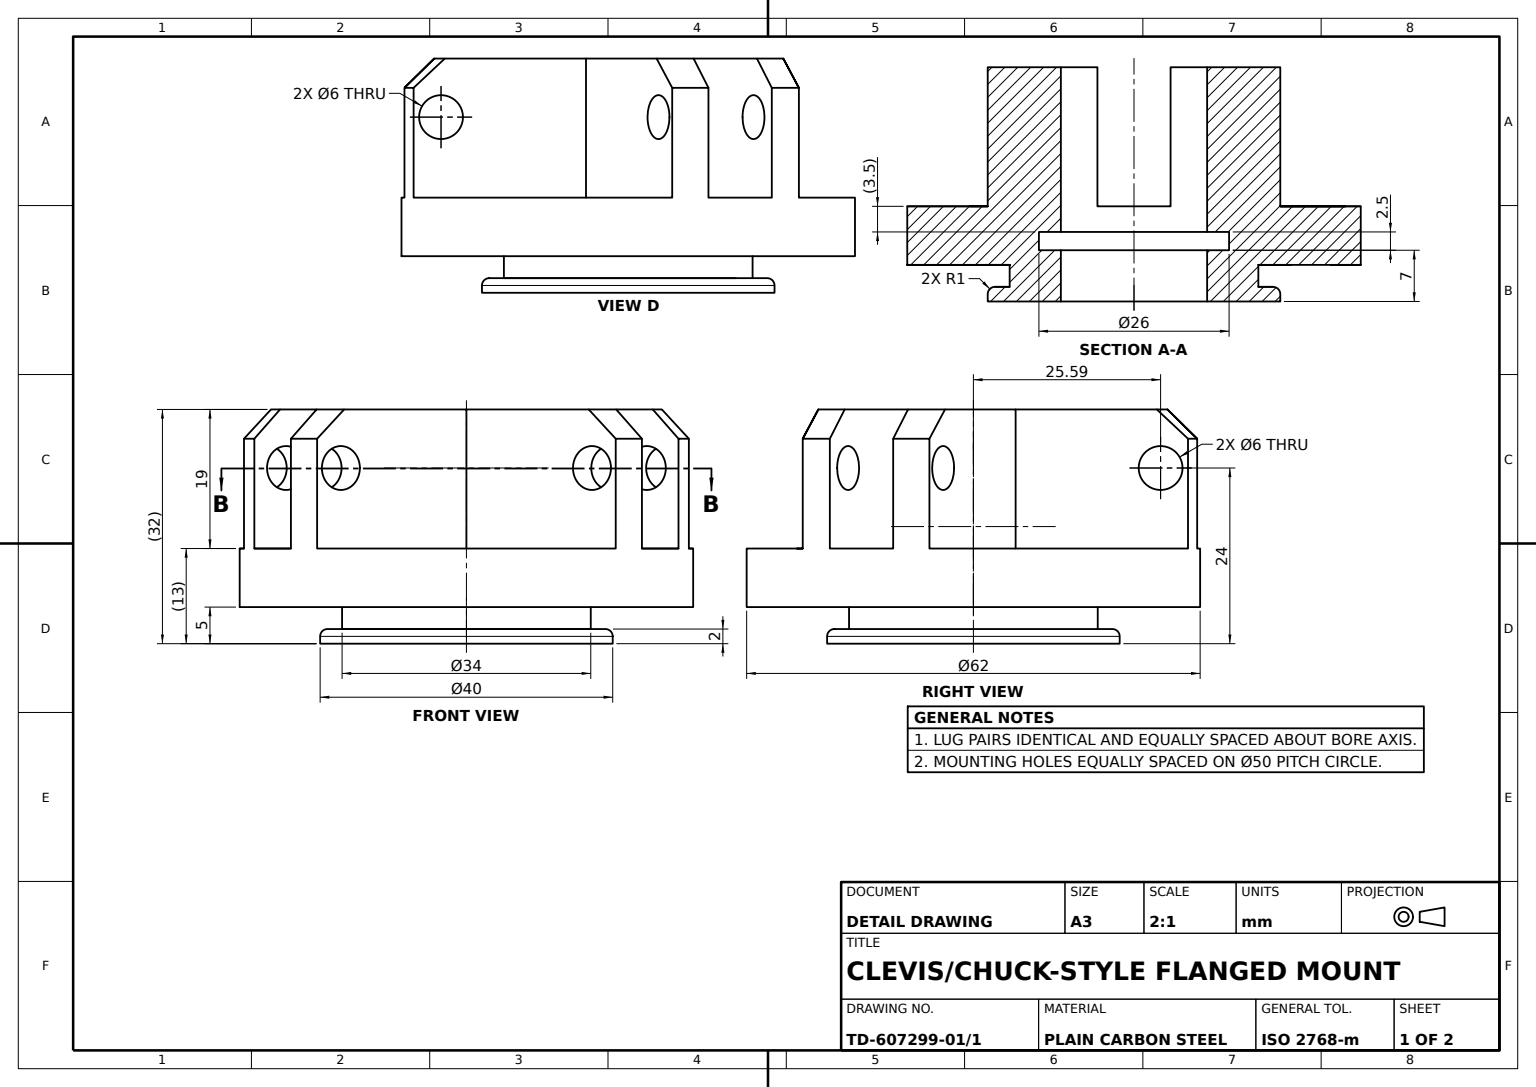
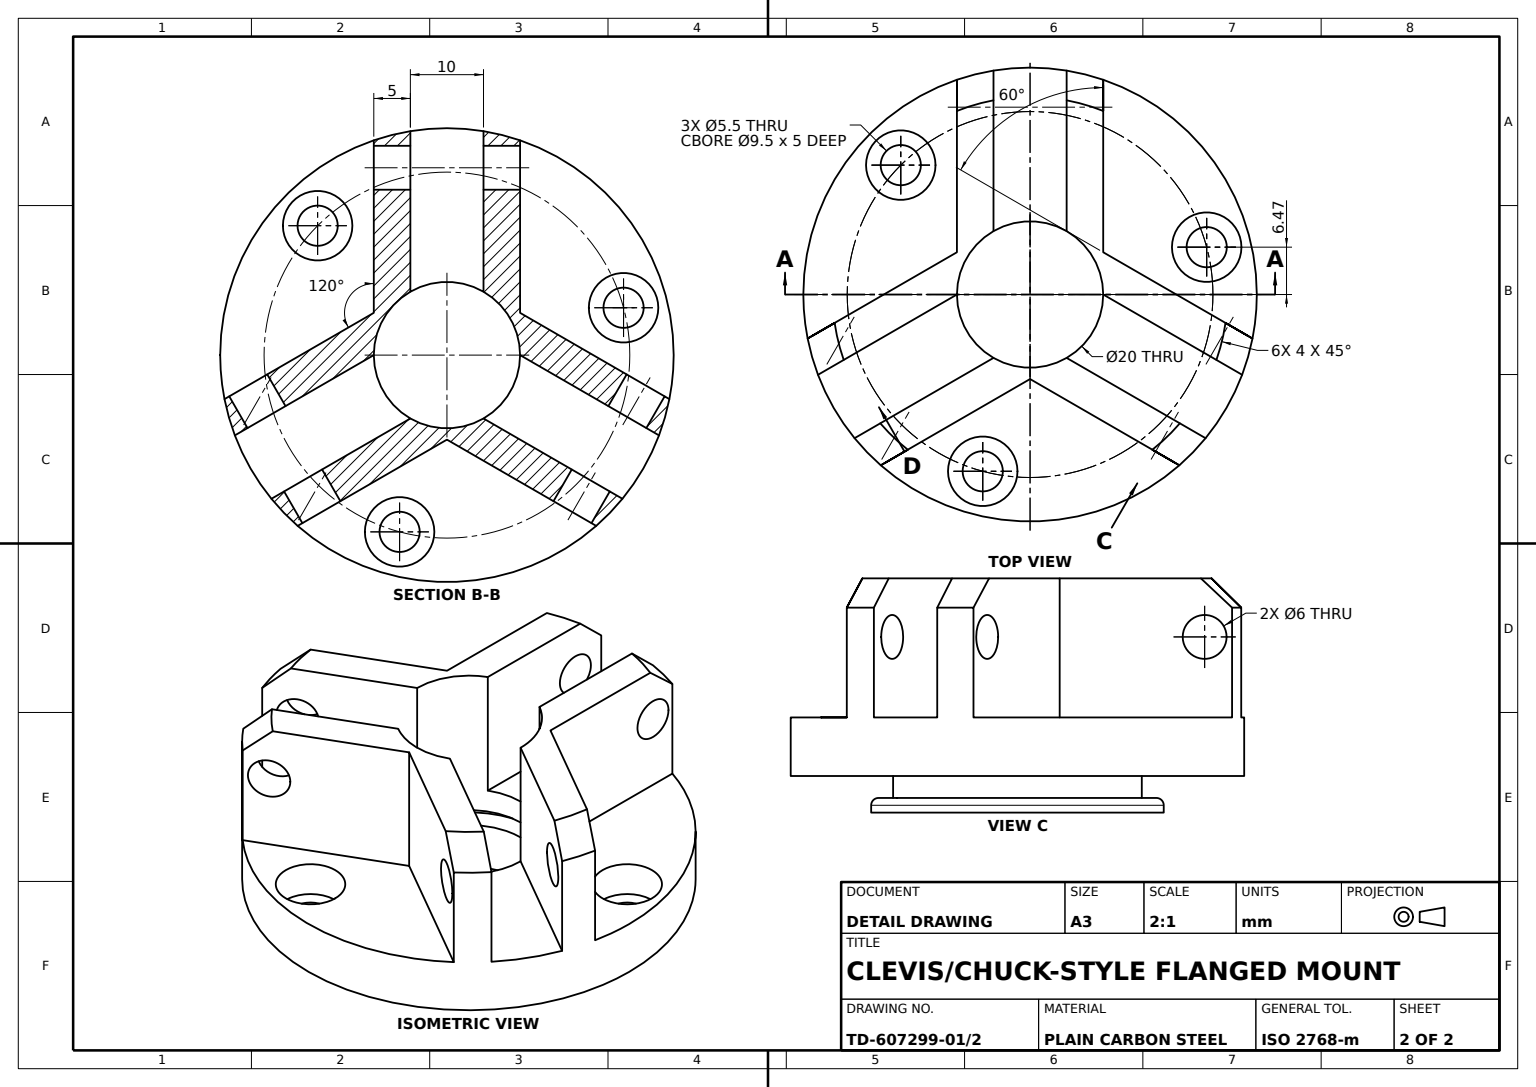
SolidWorks part; units mm, degrees
material "Plain Carbon Steel"
ref_plane "Front Plane" through (0, 0, 0) normal (0, 0, 1) x (1, 0, 0)
ref_plane "Top Plane" through (0, 0, 0) normal (0, 1, 0) x (1, 0, 0)
ref_plane "Right Plane" through (0, 0, 0) normal (1, 0, 0) x (0, 0, -1)
sketch "Base Flange Profile" plane through (0, 0, 0) normal (0, 0, 1) x (1, 0, 0)
  line L0 (0, 39.5397) -> (0, -9) construction
  line L1 (-67.2754, 0) -> (68.3671, 0) construction
  line L2 (-31, 4) -> (-31, -4)
  line L3 (-31, -4) -> (-17, -4)
  line L4 (-17, -4) -> (-17, -7)
  line L5 (-17, -7) -> (-19, -7)
  line L6 (-20, -8) -> (-20, -9)
  line L7 (-20, -9) -> (0, -9)
  line L8 (-31, 4) -> (0, 4)
  line L14 (0, 4) -> (0, -9)
  arc A0 (-20, -8) -> (-19, -7) centre (-19, -8) cw
  point P21 (-20, -7)
  dimension "D11" = 1
  dimension "D1" = 2
  dimension "D2" = 5
  dimension "D5" = 13
  dimension "D8" = 17
  dimension "D9" = 20
  dimension "D10" = 31
revolve "Base Flange Ø62" add sketch "Base Flange Profile" angle 360 about L0
sketch "Lug Profile" plane through (0, 4, 0) normal (0, 1, 0) x (1, 0, 0)
  line L0 (0, 35.3629) -> (0, 31) construction
  line L1 (0, 0) -> (37.0942, -21.4163) construction
  line L5 (5, 30.5941) -> (5, 8.6603)
  line L6 (10, 0) -> (28.9953, -10.9669)
  line L7 (10, 29.3428) -> (10, 5.7735)
  line L8 (10, 5.7735) -> (30.4116, -6.0111)
  line L9 (0, 0) -> (0, -43.2931) construction
  arc A1 (10, 0) -> (5, 8.6603) centre (0, 0) ccw
  circle A4 centre (0, 0) radius 31 construction
  arc A5 (28.9953, -10.9669) -> (30.4116, -6.0111) centre (0, 0) ccw
  arc A6 (10, 29.3428) -> (5, 30.5941) centre (0, 0) ccw
  dimension "D1" = 20
  dimension "D2" = 5
  dimension "D3" = 60
  dimension "D4" = 5
  dimension "D5" = 5
extrude "Lug" add sketch "Lug Profile" along normal blind 19
sketch "Lug Pin Hole A Sketch" plane through (5, 0, 0) normal (-1, 0, 0) x (0, 0, 1)
  line L0 (-20, -9) -> (20, -9) construction
  line L1 (-30.5941, 23) -> (-30.5941, 4) construction
  circle A0 centre (-25.5941, 15) radius 3
  dimension "D2" = 6
  dimension "D1" = 24
  dimension "D3" = 5
extrude "Lug Pin Hole A Ø6" cut sketch "Lug Pin Hole A Sketch" against normal blind 19
sketch "Lug Pin Hole B Sketch" plane through (2.5, 0, -4.3301) normal (-0.5, 0, 0.866) x (0.866, 0, 0.5)
  line L1 (-20, -9) -> (20, -9) construction
  line L2 (30.5941, 23) -> (30.5941, 4) construction
  circle A0 centre (25.5941, 15) radius 3
  dimension "D1" = 6
  dimension "D2" = 24
  dimension "D3" = 5
extrude "Lug Pin Hole B Ø6" cut sketch "Lug Pin Hole B Sketch" against normal blind 19
pattern_circular "Lug Pattern 3x120°" count 3 every 120 about axis through (0, 0, 0) along (0, 1, 0) of "Lug", "Lug Pin Hole A Ø6", "Lug Pin Hole B Ø6"
chamfer "Lug Chamfer 4mm" distance 4 angle 45 6 edges at (29.8066, 23, 8.5185) (7.5261, 23, -30.0726) (-7.5261, 23, -30.0726) (-29.8066, 23, 8.5185) (-22.2806, 23, 21.554) (22.2806, 23, 21.554)
sketch "Bore Recess Sketch" plane through (0, 4, 0) normal (0, 1, 0) x (1, 0, 0)
  circle A0 centre (0, 0) radius 10
  dimension "D1" = 20
extrude "Bore Recess Ø20 x3.5" cut sketch "Bore Recess Sketch" against normal blind 3.5
sketch "Centre Bore Sketch" plane through (0, -9, 0) normal (0, -1, 0) x (1, 0, 0)
  circle A0 centre (0, 0) radius 10
  dimension "D1" = 20
extrude "Centre Bore Ø20 x7" cut sketch "Centre Bore Sketch" against normal blind 7
sketch "Counterbore Sketch" plane through (0, -2, 0) normal (0, -1, 0) x (1, 0, 0)
  circle A0 centre (0, 0) radius 13
  dimension "D1" = 26
extrude "Counterbore Ø26 x2.5" cut sketch "Counterbore Sketch" against normal blind 2.5
sketch "Radial Slot Profile" plane through (0, 4, 0) normal (0, 1, 0) x (1, 0, 0)
  line L0 (0, 0) -> (0, -32.585) construction
  line L1 (0, 0) -> (-8.6787, -32.3895) construction
  circle A0 centre (0, 0) radius 25 construction
  circle A1 centre (-6.4705, -24.1481) radius 4.75
  dimension "D2" = 50
  dimension "D3" = 9.5
  dimension "D1" = 15
extrude "Radial Slot" cut sketch "Radial Slot Profile" against normal blind 5
sketch "Flange Hole Sketch" plane through (0, -1, 0) normal (0, 1, 0) x (1, 0, 0)
  circle A0 centre (-6.4705, -24.1481) radius 2.75
  dimension "D1" = 5.5
extrude "Flange Hole Ø5.5" cut sketch "Flange Hole Sketch" against normal through all
pattern_circular "Slot and Hole Pattern 3x120°" count 3 every 120 about axis through (0, 0, 0) along (0, 1, 0) of "Radial Slot", "Flange Hole Ø5.5"
